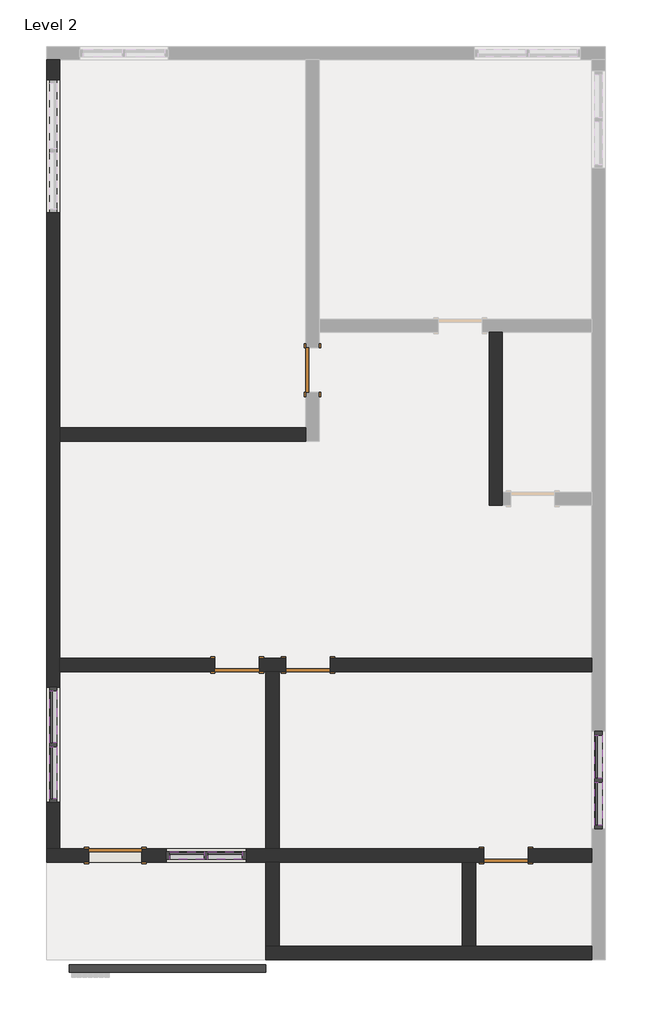
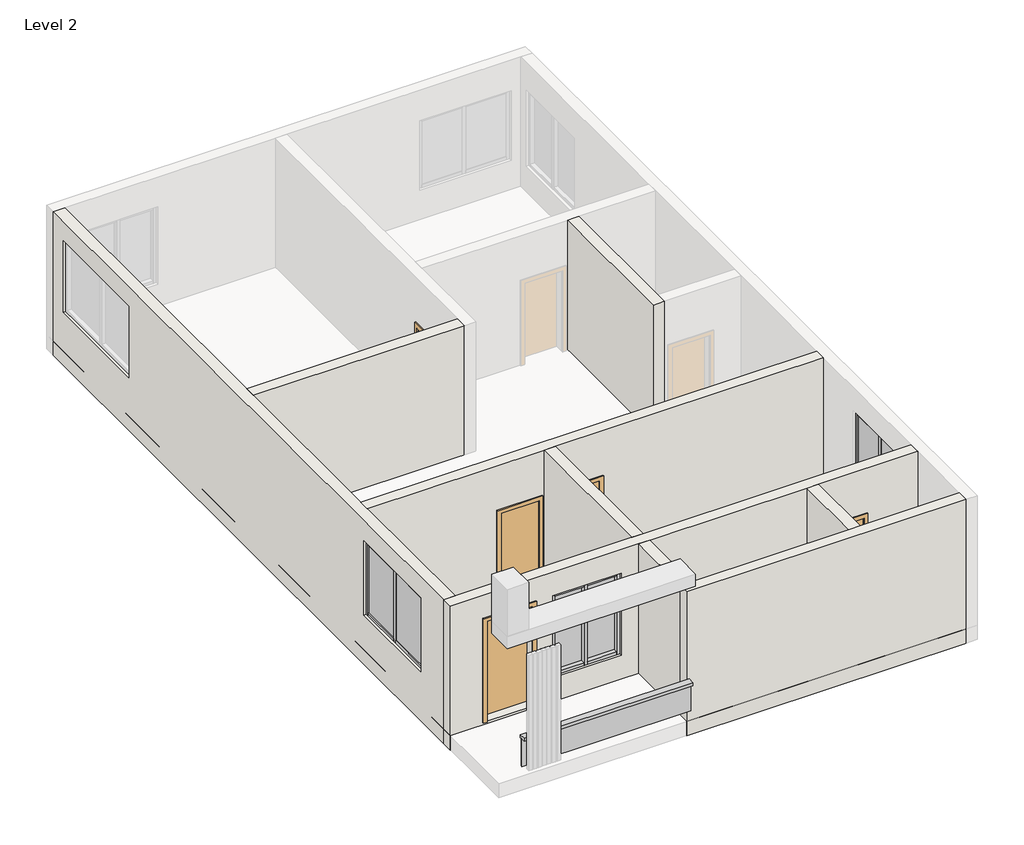
# One storey, part 1 of 2: 22 members, 9 walls, 7 plates, 5 doors.
"""IFC4 building model written with IfcOpenShell, lengths in millimetres."""

from ifc_helpers import new_model, si_unit, frame, origin, place, context, project, spatial, polyline, outline, extrude, faceted_brep, transform, mapped, element, save
from components import door_85036156, door_a1484949, door_a90ba1ad, member_e5d39754, member_064e5e56, member_82128145, member_3a0a7659, member_1e0be150, member_8ed2a5b7, member_f1f71bde, member_2820fca8, member_acc0cca9, member_6024fe87, system_panel_glazed_b741adec, system_panel_glazed_21f1ffe3, system_panel_glazed_27a553ef, system_panel_glazed_f75d5544

model = new_model("IFC4")

# Units and contexts
model_context = context("Model", 3, world=origin())
ifc_project = project(units=[si_unit("LENGTHUNIT", "METRE", prefix="MILLI")], contexts=[model_context])

# Site, building, storey
site = spatial("IfcSite", under=ifc_project)
building = spatial("IfcBuilding", under=site)
storey = spatial("IfcBuildingStorey", under=building, Name="Level 2", Elevation=3048.0)

# Doors
placement = place(None, origin())
door_shape = door_85036156(model_context)
element("IfcDoor", 1, ObjectType="Single-Flush : 30\" x 80\"", at=placement, inside=storey, context=model_context, shape_type="MappedRepresentation", body=[
    mapped(door_shape, transform((-12598.829521, -9273.5001929, 3048.0), x_axis=(1.0, 0.0, 0.0), y_axis=(0.0, 1.0, 0.0), z_axis=(0.0, 0.0, 1.0))),
])
door_2_shape = door_a1484949(model_context)
element("IfcDoor", 2, ObjectType="Single-Flush : 30\" x 80\"", at=placement, inside=storey, context=model_context, shape_type="MappedRepresentation", body=[
    mapped(door_2_shape, transform((-11379.629521, -9273.5001929, 3048.0), x_axis=(-1.0, 0.0, 0.0), y_axis=(0.0, -1.0, 0.0), z_axis=(0.0, 0.0, 1.0))),
])
element("IfcDoor", 3, ObjectType="Single-Flush : 30\" x 80\"", at=placement, inside=storey, context=model_context, shape_type="MappedRepresentation", body=[
    mapped(door_2_shape, transform((-7976.029521, -12550.1001929, 3048.0), x_axis=(-1.0, 0.0, 0.0), y_axis=(0.0, -1.0, 0.0), z_axis=(0.0, 0.0, 1.0))),
])
element("IfcDoor", 4, ObjectType="Single-Flush : 30\" x 80\"", at=placement, inside=storey, context=model_context, shape_type="MappedRepresentation", body=[
    mapped(door_2_shape, transform((-11303.429521, -4206.2001929, 3048.0), x_axis=(0.0, 1.0, 0.0), y_axis=(-1.0, 0.0, 0.0), z_axis=(0.0, 0.0, 1.0))),
])
door_3_shape = door_a90ba1ad(model_context)
element("IfcDoor", 5, ObjectType="Single-Flush : 36\" x 84\"", at=placement, inside=storey, context=model_context, shape_type="MappedRepresentation", body=[
    mapped(door_3_shape, transform((-14694.329521, -12550.1001929, 3403.6), x_axis=(-1.0, 0.0, 0.0), y_axis=(0.0, -1.0, 0.0), z_axis=(0.0, 0.0, 1.0))),
])

# Members
member_shape = member_e5d39754(model_context)
element("IfcMember", 6, ObjectType="Rectangular Mullion : 2.5\" x 5\" rectangular", at=placement, inside=storey, context=model_context, shape_type="MappedRepresentation", body=[
    mapped(member_shape, transform((-13163.979521, -12550.1001929, 5594.0897089), x_axis=(0.0, 0.0, 1.0), y_axis=(0.0, -1.0, 0.0), z_axis=(1.0, 0.0, 0.0))),
])
element("IfcMember", 7, ObjectType="Rectangular Mullion : 2.5\" x 5\" rectangular", at=placement, inside=storey, context=model_context, shape_type="MappedRepresentation", body=[
    mapped(member_shape, transform((-12509.929521, -12550.1001929, 5594.0897089), x_axis=(0.0, 0.0, 1.0), y_axis=(0.0, -1.0, 0.0), z_axis=(1.0, 0.0, 0.0))),
])
member_2_shape = member_064e5e56(model_context)
element("IfcMember", 8, ObjectType="Rectangular Mullion : 2.5\" x 5\" rectangular", at=placement, inside=storey, context=model_context, shape_type="MappedRepresentation", body=[
    mapped(member_2_shape, transform((-13132.229521, -12550.1001929, 3857.9365624), x_axis=(1.0, 0.0, 0.0), y_axis=(0.0, -1.0, 0.0), z_axis=(0.0, 0.0, -1.0))),
])
element("IfcMember", 9, ObjectType="Rectangular Mullion : 2.5\" x 5\" rectangular", at=placement, inside=storey, context=model_context, shape_type="MappedRepresentation", body=[
    mapped(member_shape, transform((-13100.479521, -12550.1001929, 3857.9365624), x_axis=(0.0, 0.0, -1.0), y_axis=(0.0, -1.0, 0.0), z_axis=(-1.0, 0.0, 0.0))),
])
element("IfcMember", 10, ObjectType="Rectangular Mullion : 2.5\" x 5\" rectangular", at=placement, inside=storey, context=model_context, shape_type="MappedRepresentation", body=[
    mapped(member_shape, transform((-13754.529521, -12550.1001929, 3857.9365624), x_axis=(0.0, 0.0, -1.0), y_axis=(0.0, -1.0, 0.0), z_axis=(-1.0, 0.0, 0.0))),
])
member_3_shape = member_82128145(model_context)
element("IfcMember", 11, ObjectType="Rectangular Mullion : 2.5\" x 5\" rectangular", at=placement, inside=storey, context=model_context, shape_type="MappedRepresentation", body=[
    mapped(member_3_shape, transform((-12446.429521, -12550.1001929, 3857.9365624), x_axis=(1.0, 0.0, 0.0), y_axis=(0.0, -1.0, 0.0), z_axis=(0.0, 0.0, -1.0))),
])
element("IfcMember", 12, ObjectType="Rectangular Mullion : 2.5\" x 5\" rectangular", at=placement, inside=storey, context=model_context, shape_type="MappedRepresentation", body=[
    mapped(member_3_shape, transform((-13818.029521, -12550.1001929, 5594.0897089), x_axis=(-1.0, 0.0, 0.0), y_axis=(0.0, -1.0, 0.0), z_axis=(0.0, 0.0, 1.0))),
])
member_4_shape = member_3a0a7659(model_context)
element("IfcMember", 13, ObjectType="Rectangular Mullion : 2.5\" x 5\" rectangular", at=placement, inside=storey, context=model_context, shape_type="MappedRepresentation", body=[
    mapped(member_4_shape, transform((-6388.529521, -11286.4501929, 5595.2359655), x_axis=(0.0, 0.0, 1.0), y_axis=(1.0, 0.0, 0.0), z_axis=(0.0, 1.0, 0.0))),
])
element("IfcMember", 14, ObjectType="Rectangular Mullion : 2.5\" x 5\" rectangular", at=placement, inside=storey, context=model_context, shape_type="MappedRepresentation", body=[
    mapped(member_4_shape, transform((-6388.529521, -10480.0001929, 5595.2359655), x_axis=(0.0, 0.0, 1.0), y_axis=(1.0, 0.0, 0.0), z_axis=(0.0, 1.0, 0.0))),
])
member_5_shape = member_1e0be150(model_context)
element("IfcMember", 15, ObjectType="Rectangular Mullion : 2.5\" x 5\" rectangular", at=placement, inside=storey, context=model_context, shape_type="MappedRepresentation", body=[
    mapped(member_5_shape, transform((-6388.529521, -11254.7001929, 3941.2993086), x_axis=(0.0, 1.0, 0.0), y_axis=(1.0, 0.0, 0.0), z_axis=(0.0, 0.0, -1.0))),
])
element("IfcMember", 16, ObjectType="Rectangular Mullion : 2.5\" x 5\" rectangular", at=placement, inside=storey, context=model_context, shape_type="MappedRepresentation", body=[
    mapped(member_4_shape, transform((-6388.529521, -11222.9501929, 3941.2993086), x_axis=(0.0, 0.0, -1.0), y_axis=(1.0, 0.0, 0.0), z_axis=(0.0, -1.0, 0.0))),
])
element("IfcMember", 17, ObjectType="Rectangular Mullion : 2.5\" x 5\" rectangular", at=placement, inside=storey, context=model_context, shape_type="MappedRepresentation", body=[
    mapped(member_4_shape, transform((-6388.529521, -12029.4001929, 3941.2993086), x_axis=(0.0, 0.0, -1.0), y_axis=(1.0, 0.0, 0.0), z_axis=(0.0, -1.0, 0.0))),
])
member_6_shape = member_8ed2a5b7(model_context)
element("IfcMember", 18, ObjectType="Rectangular Mullion : 2.5\" x 5\" rectangular", at=placement, inside=storey, context=model_context, shape_type="MappedRepresentation", body=[
    mapped(member_6_shape, transform((-6388.529521, -10416.5001929, 3941.2993086), x_axis=(0.0, 1.0, 0.0), y_axis=(1.0, 0.0, 0.0), z_axis=(0.0, 0.0, -1.0))),
])
element("IfcMember", 19, ObjectType="Rectangular Mullion : 2.5\" x 5\" rectangular", at=placement, inside=storey, context=model_context, shape_type="MappedRepresentation", body=[
    mapped(member_6_shape, transform((-6388.529521, -12092.9001929, 5595.2359655), x_axis=(0.0, -1.0, 0.0), y_axis=(1.0, 0.0, 0.0), z_axis=(0.0, 0.0, 1.0))),
])
member_7_shape = member_f1f71bde(model_context)
element("IfcMember", 20, ObjectType="Rectangular Mullion : 2.5\" x 5\" rectangular", at=placement, inside=storey, context=model_context, shape_type="MappedRepresentation", body=[
    mapped(member_7_shape, transform((-15761.129521, -10676.8501929, 5653.9047342), x_axis=(0.0, 0.0, 1.0), y_axis=(1.0, 0.0, 0.0), z_axis=(0.0, 1.0, 0.0))),
])
element("IfcMember", 21, ObjectType="Rectangular Mullion : 2.5\" x 5\" rectangular", at=placement, inside=storey, context=model_context, shape_type="MappedRepresentation", body=[
    mapped(member_7_shape, transform((-15761.129521, -9718.0001929, 5653.9047342), x_axis=(0.0, 0.0, 1.0), y_axis=(1.0, 0.0, 0.0), z_axis=(0.0, 1.0, 0.0))),
])
member_8_shape = member_2820fca8(model_context)
element("IfcMember", 22, ObjectType="Rectangular Mullion : 2.5\" x 5\" rectangular", at=placement, inside=storey, context=model_context, shape_type="MappedRepresentation", body=[
    mapped(member_8_shape, transform((-15761.129521, -10645.1001929, 4083.4359822), x_axis=(0.0, 1.0, 0.0), y_axis=(1.0, 0.0, 0.0), z_axis=(0.0, 0.0, -1.0))),
])
element("IfcMember", 23, ObjectType="Rectangular Mullion : 2.5\" x 5\" rectangular", at=placement, inside=storey, context=model_context, shape_type="MappedRepresentation", body=[
    mapped(member_7_shape, transform((-15761.129521, -10613.3501929, 4083.4359822), x_axis=(0.0, 0.0, -1.0), y_axis=(1.0, 0.0, 0.0), z_axis=(0.0, -1.0, 0.0))),
])
element("IfcMember", 24, ObjectType="Rectangular Mullion : 2.5\" x 5\" rectangular", at=placement, inside=storey, context=model_context, shape_type="MappedRepresentation", body=[
    mapped(member_7_shape, transform((-15761.129521, -11572.2001929, 4083.4359822), x_axis=(0.0, 0.0, -1.0), y_axis=(1.0, 0.0, 0.0), z_axis=(0.0, -1.0, 0.0))),
])
member_9_shape = member_acc0cca9(model_context)
element("IfcMember", 25, ObjectType="Rectangular Mullion : 2.5\" x 5\" rectangular", at=placement, inside=storey, context=model_context, shape_type="MappedRepresentation", body=[
    mapped(member_9_shape, transform((-15761.129521, -11635.7001929, 5653.9047342), x_axis=(0.0, -1.0, 0.0), y_axis=(1.0, 0.0, 0.0), z_axis=(0.0, 0.0, 1.0))),
])
element("IfcMember", 26, ObjectType="Rectangular Mullion : 2.5\" x 5\" rectangular", at=placement, inside=storey, context=model_context, shape_type="MappedRepresentation", body=[
    mapped(member_9_shape, transform((-15761.129521, -9654.5001929, 4083.4359822), x_axis=(0.0, 1.0, 0.0), y_axis=(1.0, 0.0, 0.0), z_axis=(0.0, 0.0, -1.0))),
])
member_10_shape = member_6024fe87(model_context)
element("IfcMember", 27, ObjectType="Rectangular Mullion : 2.5\" x 5\" rectangular", at=placement, inside=storey, context=model_context, shape_type="MappedRepresentation", body=[
    mapped(member_10_shape, transform((-12103.529521, -14493.2001929, 4306.1687666), x_axis=(0.0, 0.0, 1.0), y_axis=(0.0, -1.0, 0.0), z_axis=(1.0, 0.0, 0.0))),
])

# Plates
system_panel_glazed_shape = system_panel_glazed_b741adec(model_context)
element("IfcPlate", 28, ObjectType="System Panel : Glazed", at=placement, inside=storey, context=model_context, shape_type="MappedRepresentation", body=[
    mapped(system_panel_glazed_shape, transform((-13459.254521, -12550.1001929, 3921.4365624), x_axis=(1.0, 0.0, 0.0), y_axis=(0.0, 1.0, 0.0), z_axis=(0.0, 0.0, 1.0))),
])
element("IfcPlate", 29, ObjectType="System Panel : Glazed", at=placement, inside=storey, context=model_context, shape_type="MappedRepresentation", body=[
    mapped(system_panel_glazed_shape, transform((-12805.204521, -12550.1001929, 3921.4365624), x_axis=(1.0, 0.0, 0.0), y_axis=(0.0, 1.0, 0.0), z_axis=(0.0, 0.0, 1.0))),
])
system_panel_glazed_2_shape = system_panel_glazed_21f1ffe3(model_context)
element("IfcPlate", 30, ObjectType="System Panel : Glazed", at=placement, inside=storey, context=model_context, shape_type="MappedRepresentation", body=[
    mapped(system_panel_glazed_2_shape, transform((-6388.529521, -11657.9251929, 4004.7993086), x_axis=(0.0, 1.0, 0.0), y_axis=(-1.0, 0.0, 0.0), z_axis=(0.0, 0.0, 1.0))),
])
element("IfcPlate", 31, ObjectType="System Panel : Glazed", at=placement, inside=storey, context=model_context, shape_type="MappedRepresentation", body=[
    mapped(system_panel_glazed_2_shape, transform((-6388.529521, -10851.4751929, 4004.7993086), x_axis=(0.0, 1.0, 0.0), y_axis=(-1.0, 0.0, 0.0), z_axis=(0.0, 0.0, 1.0))),
])
system_panel_glazed_3_shape = system_panel_glazed_27a553ef(model_context)
element("IfcPlate", 32, ObjectType="System Panel : Glazed", at=placement, inside=storey, context=model_context, shape_type="MappedRepresentation", body=[
    mapped(system_panel_glazed_3_shape, transform((-15761.129521, -11124.5251929, 4146.9359822), x_axis=(0.0, 1.0, 0.0), y_axis=(-1.0, 0.0, 0.0), z_axis=(0.0, 0.0, 1.0))),
])
element("IfcPlate", 33, ObjectType="System Panel : Glazed", at=placement, inside=storey, context=model_context, shape_type="MappedRepresentation", body=[
    mapped(system_panel_glazed_3_shape, transform((-15761.129521, -10165.6751929, 4146.9359822), x_axis=(0.0, 1.0, 0.0), y_axis=(-1.0, 0.0, 0.0), z_axis=(0.0, 0.0, 1.0))),
])
system_panel_glazed_4_shape = system_panel_glazed_f75d5544(model_context)
element("IfcPlate", 34, ObjectType="System Panel : Glazed", at=placement, inside=storey, context=model_context, shape_type="MappedRepresentation", body=[
    mapped(system_panel_glazed_4_shape, transform((-13795.5232683, -14493.2001929, 3657.6), x_axis=(1.0, 0.0, 0.0), y_axis=(0.0, 1.0, 0.0), z_axis=(0.0, 0.0, 1.0))),
])

# Walls
element("IfcWall", 35, ObjectType="9\"", at=placement, inside=storey, context=model_context, shape_type="Brep", body=[
    faceted_brep([(-6502.829521, -14112.2001929, 3048.0), (-8496.729521, -14112.2001929, 3048.0), (-8725.329521, -14112.2001929, 3048.0), (-11874.929521, -14112.2001929, 3048.0), (-12103.529521, -14112.2001929, 3048.0), (-12103.529521, -14112.2001929, 6096.0), (-11874.929521, -14112.2001929, 6096.0), (-8725.329521, -14112.2001929, 6096.0), (-8496.729521, -14112.2001929, 6096.0), (-6502.829521, -14112.2001929, 6096.0), (-6502.829521, -14340.8001929, 3048.0), (-6502.829521, -14340.8001929, 6096.0), (-12103.529521, -14340.8001929, 6096.0), (-12103.529521, -14340.8001929, 3048.0)], [[[0, 1, 2, 3, 4, 5, 6, 7, 8, 9]], [[10, 11, 12, 13]], [[4, 3, 2, 1, 0, 10, 13]], [[9, 8, 7, 6, 5, 12, 11]], [[0, 9, 11, 10]], [[5, 4, 13, 12]]]),
])
element("IfcWall", 36, ObjectType="9\"", at=placement, inside=storey, context=model_context, shape_type="SweptSolid", body=[
    extrude(outline(polyline([(-11874.929521, -12664.4001929), (-11874.929521, -14112.2001929), (-12103.529521, -14112.2001929), (-12103.529521, -12664.4001929), (-11874.929521, -12664.4001929)])), frame((0.0, 0.0, 3048.0), z_axis=(0.0, 0.0, 1.0), x_axis=(1.0, 0.0, 0.0)), (0.0, 0.0, 1.0), 3048.0),
])
element("IfcWall", 37, ObjectType="9\"", at=placement, inside=storey, context=model_context, shape_type="Brep", body=[
    faceted_brep([(-15875.429521, -12435.8001929, 6096.0), (-15646.829521, -12435.8001929, 6096.0), (-12103.529521, -12435.8001929, 6096.0), (-11874.929521, -12435.8001929, 6096.0), (-6502.829521, -12435.8001929, 6096.0), (-6502.829521, -12435.8001929, 3048.0), (-7595.029521, -12435.8001929, 3048.0), (-7595.029521, -12435.8001929, 5080.0), (-8357.029521, -12435.8001929, 5080.0), (-8357.029521, -12435.8001929, 3048.0), (-11874.929521, -12435.8001929, 3048.0), (-12103.529521, -12435.8001929, 3048.0), (-15646.829521, -12435.8001929, 3048.0), (-15875.429521, -12435.8001929, 3048.0), (-15151.529521, -12435.8001929, 3403.6), (-14237.129521, -12435.8001929, 3403.6), (-14237.129521, -12435.8001929, 5537.2), (-15151.529521, -12435.8001929, 5537.2), (-13818.029521, -12435.8001929, 5594.0897089), (-13818.029521, -12435.8001929, 3857.9365624), (-12446.429521, -12435.8001929, 3857.9365624), (-12446.429521, -12435.8001929, 5594.0897089), (-6502.829521, -12664.4001929, 6096.0), (-8496.729521, -12664.4001929, 6096.0), (-8725.329521, -12664.4001929, 6096.0), (-11874.929521, -12664.4001929, 6096.0), (-12103.529521, -12664.4001929, 6096.0), (-15875.429521, -12664.4001929, 6096.0), (-15875.429521, -12664.4001929, 3048.0), (-12103.529521, -12664.4001929, 3048.0), (-11874.929521, -12664.4001929, 3048.0), (-8725.329521, -12664.4001929, 3048.0), (-8496.729521, -12664.4001929, 3048.0), (-8357.029521, -12664.4001929, 3048.0), (-8357.029521, -12664.4001929, 5080.0), (-7595.029521, -12664.4001929, 5080.0), (-7595.029521, -12664.4001929, 3048.0), (-6502.829521, -12664.4001929, 3048.0), (-14237.129521, -12664.4001929, 3403.6), (-15151.529521, -12664.4001929, 3403.6), (-15151.529521, -12664.4001929, 5537.2), (-14237.129521, -12664.4001929, 5537.2), (-13818.029521, -12664.4001929, 3857.9365624), (-13818.029521, -12664.4001929, 5594.0897089), (-12446.429521, -12664.4001929, 5594.0897089), (-12446.429521, -12664.4001929, 3857.9365624)], [[[0, 1, 2, 3, 4, 5, 6, 7, 8, 9, 10, 11, 12, 13], [14, 15, 16, 17], [18, 19, 20, 21]], [[22, 23, 24, 25, 26, 27, 28, 29, 30, 31, 32, 33, 34, 35, 36, 37], [38, 39, 40, 41], [42, 43, 44, 45]], [[28, 13, 12, 11, 10, 9, 33, 32, 31, 30, 29]], [[5, 37, 36, 6]], [[4, 3, 2, 1, 0, 27, 26, 25, 24, 23, 22]], [[0, 13, 28, 27]], [[5, 4, 22, 37]], [[39, 38, 15, 14]], [[40, 39, 14, 17]], [[41, 40, 17, 16]], [[38, 41, 16, 15]], [[34, 33, 9, 8]], [[35, 34, 8, 7]], [[36, 35, 7, 6]], [[42, 19, 18, 43]], [[43, 18, 21, 44]], [[44, 21, 20, 45]], [[19, 42, 45, 20]]]),
])
element("IfcWall", 38, ObjectType="9\"", at=placement, inside=storey, context=model_context, shape_type="Brep", body=[
    faceted_brep([(-15875.429521, 1127.7998071, 3048.0), (-15875.429521, -12435.8001929, 3048.0), (-15875.429521, -12435.8001929, 6096.0), (-15875.429521, 1127.7998071, 6096.0), (-15875.429521, -11635.7001929, 5653.9047342), (-15875.429521, -11635.7001929, 4083.4359822), (-15875.429521, -9654.5001929, 4083.4359822), (-15875.429521, -9654.5001929, 5653.9047342), (-15875.429521, 784.8998071, 4168.4028546), (-15875.429521, 784.8998071, 5689.5924867), (-15875.429521, -1501.1001929, 5689.5924867), (-15875.429521, -1501.1001929, 4168.4028546), (-15646.829521, -12435.8001929, 3048.0), (-15646.829521, -9387.8001929, 3048.0), (-15646.829521, -9159.2001929, 3048.0), (-15646.829521, -5425.4001929, 3048.0), (-15646.829521, -5196.8001929, 3048.0), (-15646.829521, 1127.7998071, 3048.0), (-15646.829521, 1127.7998071, 6096.0), (-15646.829521, -5196.8001929, 6096.0), (-15646.829521, -5425.4001929, 6096.0), (-15646.829521, -9159.2001929, 6096.0), (-15646.829521, -9387.8001929, 6096.0), (-15646.829521, -12435.8001929, 6096.0), (-15646.829521, -11635.7001929, 4083.4359822), (-15646.829521, -11635.7001929, 5653.9047342), (-15646.829521, -9654.5001929, 5653.9047342), (-15646.829521, -9654.5001929, 4083.4359822), (-15646.829521, 784.8998071, 5689.5924867), (-15646.829521, 784.8998071, 4168.4028546), (-15646.829521, -1501.1001929, 4168.4028546), (-15646.829521, -1501.1001929, 5689.5924867)], [[[0, 1, 2, 3], [4, 5, 6, 7], [8, 9, 10, 11]], [[12, 13, 14, 15, 16, 17, 18, 19, 20, 21, 22, 23], [24, 25, 26, 27], [28, 29, 30, 31]], [[1, 0, 17, 16, 15, 14, 13, 12]], [[3, 2, 23, 22, 21, 20, 19, 18]], [[2, 1, 12, 23]], [[0, 3, 18, 17]], [[24, 5, 4, 25]], [[25, 4, 7, 26]], [[26, 7, 6, 27]], [[5, 24, 27, 6]], [[8, 29, 28, 9]], [[9, 28, 31, 10]], [[30, 11, 10, 31]], [[29, 8, 11, 30]]]),
])
element("IfcWall", 39, ObjectType="9\"", at=placement, inside=storey, context=model_context, shape_type="SweptSolid", body=[
    extrude(outline(polyline([(-11417.729521, -5425.4001929), (-15646.829521, -5425.4001929), (-15646.829521, -5196.8001929), (-11417.729521, -5196.8001929), (-11417.729521, -5425.4001929)])), frame((0.0, 0.0, 3048.0), z_axis=(0.0, 0.0, 1.0), x_axis=(1.0, 0.0, 0.0)), (0.0, 0.0, 1.0), 3048.0),
])
element("IfcWall", 40, ObjectType="9\"", at=placement, inside=storey, context=model_context, shape_type="Brep", body=[
    faceted_brep([(-8268.129521, -3558.5001929, 3048.0), (-8268.129521, -6530.3001929, 3048.0), (-8268.129521, -6530.3001929, 6096.0), (-8268.129521, -3558.5001929, 6096.0), (-8039.529521, -3558.5001929, 3048.0), (-8039.529521, -3558.5001929, 6096.0), (-8039.529521, -6301.7001929, 6096.0), (-8039.529521, -6530.3001929, 6096.0), (-8039.529521, -6530.3001929, 3048.0), (-8039.529521, -6301.7001929, 3048.0)], [[[0, 1, 2, 3]], [[4, 5, 6, 7, 8, 9]], [[1, 0, 4, 9, 8]], [[3, 2, 7, 6, 5]], [[0, 3, 5, 4]], [[2, 1, 8, 7]]]),
])
element("IfcWall", 41, ObjectType="9\"", at=placement, inside=storey, context=model_context, shape_type="SweptSolid", body=[
    extrude(outline(polyline([(-8725.329521, -14112.2001929), (-8725.329521, -12664.4001929), (-8496.729521, -12664.4001929), (-8496.729521, -14112.2001929), (-8725.329521, -14112.2001929)])), frame((0.0, 0.0, 3048.0), z_axis=(0.0, 0.0, 1.0), x_axis=(1.0, 0.0, 0.0)), (0.0, 0.0, 1.0), 3048.0),
])
element("IfcWall", 42, ObjectType="9\"", at=placement, inside=storey, context=model_context, shape_type="SweptSolid", body=[
    extrude(outline(polyline([(-11874.929521, -9387.8001929), (-11874.929521, -12435.8001929), (-12103.529521, -12435.8001929), (-12103.529521, -9387.8001929), (-11874.929521, -9387.8001929)])), frame((0.0, 0.0, 3048.0), z_axis=(0.0, 0.0, 1.0), x_axis=(1.0, 0.0, 0.0)), (0.0, 0.0, 1.0), 3048.0),
])
element("IfcWall", 43, ObjectType="9\"", at=placement, inside=storey, context=model_context, shape_type="Brep", body=[
    faceted_brep([(-11760.629521, -9159.2001929, 3048.0), (-12217.829521, -9159.2001929, 3048.0), (-12217.829521, -9159.2001929, 5080.0), (-12979.829521, -9159.2001929, 5080.0), (-12979.829521, -9159.2001929, 3048.0), (-15646.829521, -9159.2001929, 3048.0), (-15646.829521, -9159.2001929, 6096.0), (-6502.829521, -9159.2001929, 6096.0), (-6502.829521, -9159.2001929, 3048.0), (-10998.629521, -9159.2001929, 3048.0), (-10998.629521, -9159.2001929, 5080.0), (-11760.629521, -9159.2001929, 5080.0), (-12217.829521, -9387.8001929, 5080.0), (-12217.829521, -9387.8001929, 3048.0), (-12103.529521, -9387.8001929, 3048.0), (-11874.929521, -9387.8001929, 3048.0), (-11760.629521, -9387.8001929, 3048.0), (-11760.629521, -9387.8001929, 5080.0), (-10998.629521, -9387.8001929, 5080.0), (-10998.629521, -9387.8001929, 3048.0), (-6502.829521, -9387.8001929, 3048.0), (-6502.829521, -9387.8001929, 6096.0), (-11874.929521, -9387.8001929, 6096.0), (-12103.529521, -9387.8001929, 6096.0), (-15646.829521, -9387.8001929, 6096.0), (-15646.829521, -9387.8001929, 3048.0), (-12979.829521, -9387.8001929, 3048.0), (-12979.829521, -9387.8001929, 5080.0)], [[[0, 1, 2, 3, 4, 5, 6, 7, 8, 9, 10, 11]], [[12, 13, 14, 15, 16, 17, 18, 19, 20, 21, 22, 23, 24, 25, 26, 27]], [[9, 8, 20, 19]], [[26, 25, 5, 4]], [[16, 15, 14, 13, 1, 0]], [[7, 6, 24, 23, 22, 21]], [[6, 5, 25, 24]], [[8, 7, 21, 20]], [[17, 16, 0, 11]], [[18, 17, 11, 10]], [[19, 18, 10, 9]], [[2, 1, 13, 12]], [[3, 2, 12, 27]], [[4, 3, 27, 26]]]),
])

save(model, "model.ifc")

# Revit data of these elements
# Type "Single-Flush : 30\" x 80\""
#   Type Mark = "5"
#   Construction Type Id = "MDOOR"
#   Assembly Code = "C1020"
#   Analytic Construction = "Metal"
#   Thickness = 0' - 2"
#   Heat Transfer Coefficient (U) = 0.651978 BTU/(h·ft²·°F)
#   Height = 6' - 8"
#   Trim Projection Ext = 0' - 1"
#   Trim Projection Int = 0' - 1"
#   Trim Width = 0' - 3"
#   Width = 2' - 6"
#   Define Thermal Properties by = 1
#   Define Thermal Properties by = 1
#   Door Material = Door - Panel
#   Frame Material = Door - Frame
#   Visual Light Transmittance = 0
#   Solar Heat Gain Coefficient = 0
#   Function = (empty or 0)
#   Wall Closure = (empty or 0)
# Type "Single-Flush : 36\" x 84\""
#   Type Mark = "1"
#   Construction Type Id = "MDOOR"
#   Assembly Code = "C1020"
#   Analytic Construction = "Metal"
#   Thickness = 0' - 2"
#   Heat Transfer Coefficient (U) = 0.651978 BTU/(h·ft²·°F)
#   Height = 7' - 0"
#   Trim Projection Ext = 0' - 1"
#   Trim Projection Int = 0' - 1"
#   Trim Width = 0' - 3"
#   Width = 3' - 0"
#   Define Thermal Properties by = 1
#   Define Thermal Properties by = 1
#   Door Material = Door - Panel
#   Frame Material = Door - Frame
#   Visual Light Transmittance = 0
#   Solar Heat Gain Coefficient = 0
#   Function = (empty or 0)
#   Wall Closure = (empty or 0)
# Type "Rectangular Mullion : 2.5\" x 5\" rectangular"
#   built-in parameter 1007304 = 0.416667 (stored number, unit not read)
#   built-in parameter 1007301 = 0.104167 (stored number, unit not read)
#   built-in parameter 1007300 = 0.104167 (stored number, unit not read)
# Type "System Panel : Glazed"
#   Construction Type Id = "GSP4R"
#   Analytic Construction = "1/8 in Pilkington single glazing"
#   Visual Light Transmittance = 0.9
#   Solar Heat Gain Coefficient = 0.86
#   Heat Transfer Coefficient (U) = 1.18115 BTU/(h·ft²·°F)
#   Define Thermal Properties by = 1
# Type "9\""
#   Assembly Code = "B2010"
#   Layers, outside or top first: 0' - 9" no material (function 1)
# Elements 1, 2, 3, 4 (IfcDoor, "Single-Flush : 30\" x 80\"")
#   Phase Created = New Construction
#   Materials on its faces: "Door - Frame", "Door - Panel"
# Element 5 (IfcDoor, "Single-Flush : 36\" x 84\"")
#   Phase Created = New Construction
#   Materials on its faces: "Door - Frame", "Door - Panel"
# Elements 6, 7, 8, 9, 10, 11, 12, 13, 14, 15, 16, 17, 18, 19, 20, 21, 22, 23, 24, 25, 26, 27 (IfcMember, "Rectangular Mullion : 2.5\" x 5\" rectangular")
#   Phase Created = New Construction
#   Materials on its faces: "Aluminum"
# Elements 28, 29, 30, 31, 32, 33, 34 (IfcPlate, "System Panel : Glazed")
#   Phase Created = New Construction
#   Materials on its faces: "Glass"
# Elements 35, 36, 37, 38, 39, 40, 41, 42, 43 (IfcWall, "9\"")
#   Top Offset = 0' - 0"
#   Base Offset = 0' - 0"
#   Unconnected Height = 10' - 0"
#   wall height = 10' - 0"
#   Phase Created = New Construction
#   Base Constraint = Level 2
#   Materials on its faces: "Default Wall"
# Materials
#   "Door - Panel": class "Wood", colour RGB 210 159 95, transparency 0, Cost = 0
#   "Door - Frame": colour RGB 118 70 51, transparency 0, Cost = 0
#   "Aluminum": class "Metal", colour RGB 247 247 247, transparency 0, Description = "Aluminum 6061", Cost = 0
#   "Glass": class "Glass", colour RGB 0 128 192, transparency 0.75, Description = "Soda Lime Glass", Cost = 0
#   "Default Wall": colour RGB 128 128 128, transparency 0, Cost = 0
